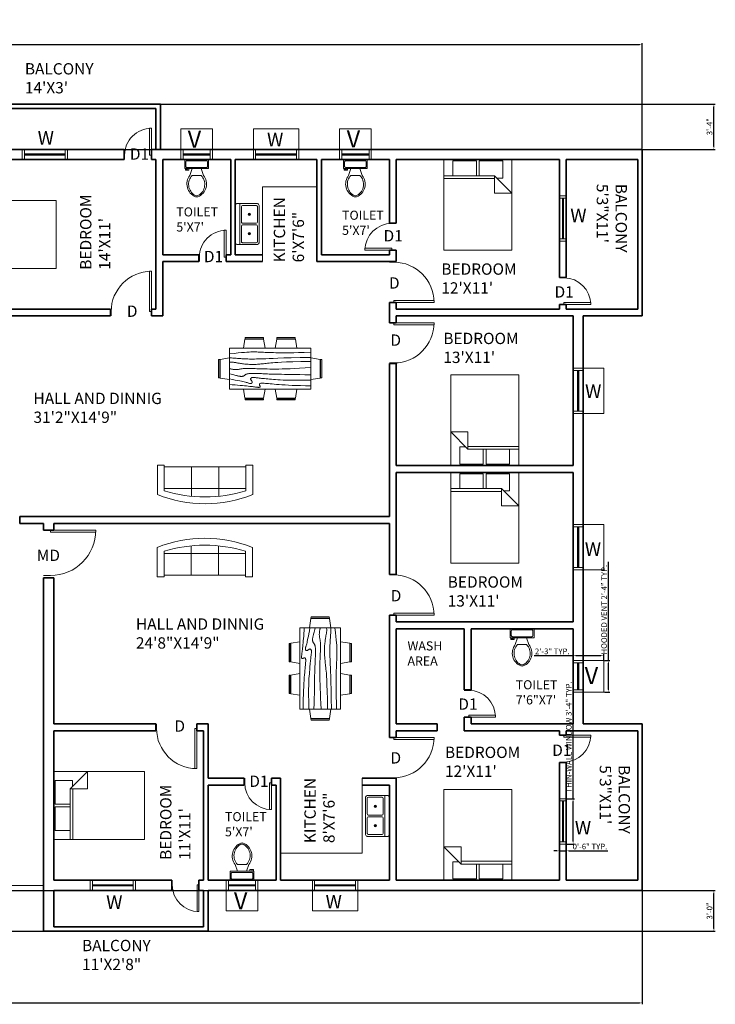
# Model space of a CAD drawing. Units: inches. Extents: x 1662 to 23131, y 1265 to 19127.
# Tile 19 of 26: x 20147 to 20761, y 18258 to 19127. Entities that reach past the tile are written whole.
import ezdxf

# ---------------------------------------------------------------- set-up
doc = ezdxf.new("R2010")
doc.units = ezdxf.units.IN
for name, color, linetype, lineweight in [('A-ANNO-DIMS', 4, 'Continuous', 18), ('A-ANNO-IDEN', 7, 'Continuous', 18), ('A-AREA-IDEN', 7, 'Continuous', 18), ('A-DOOR', 3, 'Continuous', 18), ('A-DOOR-GATE', 3, 'Continuous', 18), ('A-FLOR-CASE', 8, 'Continuous', 18), ('A-FLOR-FIXT', 9, 'Continuous', 18), ('A-FURN', 8, 'Continuous', 18), ('A-GLAZ', 4, 'Continuous', 18), ('A-WALL', 7, 'Continuous', 35)]:
    doc.layers.add(name, color=color, linetype=linetype, lineweight=lineweight)
doc.styles.get("Standard").update_dxf_attribs({"font": 'arial.ttf'})
doc.dimstyles.new('ISO-25', dxfattribs={"dimtxt": 5, "dimasz": 2.5, "dimexe": 1.25, "dimexo": 0.625, "dimtad": 1, "dimlunit": 3, "dimtxsty": 'Standard', "dimcen": 2.5, "dimadec": 0, "dimazin": 0, "dimtfac": 1, "dimtmove": 0, "dimatfit": 3, "dimfxl": 1, "dimarcsym": 0})

# ---------------------------------------------------------------- blocks, each defined once
blk = doc.blocks.new('Bed - Queen')
for p, q in [((0, -80.00003), (0, 0)), ((0, 0), (59.99999, 0)), ((59.99999, 0), (59.99999, -80.00003)), ((7.99999, -1.2), (28.79998, -1.2)), ((7.99999, -14.4), (7.99999, -1.2)), ((28.79998, -1.2), (28.79998, -14.4)), ((31.19999, -1.2), (51.99999, -1.2)), ((31.19999, -14.4), (31.19999, -1.2)), ((51.99999, -1.2), (51.99999, -16.4)), ((0, -14.4), (44.8, -14.4)), ((44.8, -16.8), (0, -16.8)), ((59.99999, -29.6), (44.8, -14.4)), ((44.8, -14.4), (44.8, -29.6)), ((51.99999, -16.4), (46.79936, -16.4)), ((44.8, -29.6), (59.99999, -29.6)), ((59.99999, -80.00003), (0, -80.00003))]:
    blk.add_line(p, q)
blk = doc.blocks.new('Toilet - top')
for p, q in [((-10, -8.5), (-8, -8.5)), ((-10, -9.5), (-10, -8.5)), ((-8, -8.5), (-8, -8)), ((-7, -8), (-7, -9.5)), ((-4, -8), (-6, -14)), ((4, -8), (6, -14)), ((9.5, -6), (9.5, -2)), ((-7, -9.5), (-10, -9.5)), ((4, -14), (-4, -14))]:
    blk.add_line(p, q)
blk.add_lwpolyline([(10.5, -8), (10.5, 0), (-10.5, 0), (-10.5, -8)], close=True)
for points in [[(-9.5, -2), (-9.5, -6)], [(8.5, -1), (-8.5, -1)], [(-8.5, -7), (8.5, -7)]]:
    blk.add_lwpolyline(points)
for centre, radius, start, end in [((-8.62, -1.88), 0.884, 81.8699, 188.1301), ((-8.62, -6.12), 0.884, 171.8699, 278.1301), ((8.62, -1.88), 0.884, 351.8699, 98.1301), ((8.62, -6.12), 0.884, 261.8699, 8.1301), ((3.52, -21.58), 12.17, 141.46911, 247.97143), ((4.2, -21.82), 11.33, 136.36773, 238.94682), ((-3.52, -21.58), 12.17, 292.02843, 38.53071), ((-4.2, -21.82), 11.33, 301.05301, 43.63209), ((0, -27.88), 4, 245.73182, 294.26817), ((0, -29), 4, 254.86053, 285.13947)]:
    blk.add_arc(centre, radius, start, end)
blk = doc.blocks.new('Sink-double - 36 in top')
for p, q in [((-18, -4), (18, -4)), ((-0.75, -18.5), (-0.75, -6.5)), ((0.75, -6.5), (0.75, -18.5))]:
    blk.add_line(p, q)
for points in [[(-16.5, 0), (16.5, 0)], [(-18, -19.5), (-18, -1.5)], [(-16.5, -18.5), (-16.5, -6.5)], [(-15.5, -5.5), (-1.75, -5.5)], [(1.75, -5.5), (15.5, -5.5)], [(16.5, -6.5), (16.5, -18.5)], [(18, -1.5), (18, -19.5)], [(16.5, -21), (-16.5, -21)], [(-1.75, -19.5), (-15.5, -19.5)], [(15.5, -19.5), (1.75, -19.5)]]:
    blk.add_lwpolyline(points)
for centre, radius in [((-8.5, -12.5), 1), ((-8.5, -12.5), 0.5), ((8.5, -12.5), 1), ((8.5, -12.5), 0.5)]:
    blk.add_circle(centre, radius)
for centre, radius, start, end in [((-16.5, -1.5), 1.5, 90, 180), ((16.5, -1.5), 1.5, 0, 90), ((-15.5, -6.5), 1, 90, 180), ((-1.75, -6.5), 1, 0, 90), ((1.75, -6.5), 1, 90, 180), ((15.5, -6.5), 1, 0, 90), ((-16.5, -19.5), 1.5, 180, 270), ((-15.5, -18.5), 1, 180, 270), ((-1.75, -18.5), 1, 270, 0), ((1.75, -18.5), 1, 180, 270), ((15.5, -18.5), 1, 270, 0), ((16.5, -19.5), 1.5, 270, 0)]:
    blk.add_arc(centre, radius, start, end)
blk = doc.blocks.new('Dining Set - 36 x 72 in.')
for p, q in [((-22, 27.5), (-22.1562, 26.50042)), ((-5.8416, 26.5), (-22.1534, 26.5)), ((-22, 27.5), (-6, 27.5)), ((-5.8437, 26.49966), (-6, 27.5)), ((6, 27.5), (5.8438, 26.50042)), ((22.1584, 26.5), (5.8466, 26.5)), ((6, 27.5), (22, 27.5)), ((22.1563, 26.49966), (22, 27.5)), ((36, 18), (-36, 18)), ((-36, 18), (-36, -18)), ((-22.2343, 26.00059), (-23.4847, 17.99762)), ((-22.2304, 26), (-5.7608, 26)), ((-4.5152, 17.99762), (-5.7655, 25.99926)), ((5.7657, 26.00059), (4.5153, 17.99762)), ((5.7696, 26), (22.2392, 26)), ((23.4848, 17.99762), (22.2345, 25.99926)), ((36, -18), (36, 18)), ((-44.0006, 8.23428), (-35.9976, 9.48474)), ((44.0006, 8.23428), (35.9976, 9.48474)), ((-45.5, 8), (-44.5004, 8.15617)), ((-45.5, 8), (-45.5, -8)), ((-44.5, -8.15843), (-44.5, 8.15338)), ((-44, 8.23041), (-44, -8.23915)), ((44, 8.23041), (44, -8.23915)), ((44.5, -8.15843), (44.5, 8.15338)), ((45.5, 8), (44.5005, 8.15617)), ((45.5, 8), (45.5, -8)), ((-44.4997, -8.15631), (-45.5, -8)), ((-35.9976, -9.48476), (-43.9993, -8.2345)), ((35.9976, -9.48476), (43.9993, -8.2345)), ((44.4997, -8.15631), (45.5, -8)), ((-36, -18), (36, -18)), ((-22.2343, -26.0006), (-23.4847, -17.99762)), ((-22.2304, -26), (-5.7608, -26)), ((-4.5152, -17.99762), (-5.7655, -25.99928)), ((5.7657, -26.0006), (4.5153, -17.99762)), ((5.7696, -26), (22.2392, -26)), ((23.4848, -17.99762), (22.2345, -25.99928)), ((-22, -27.5), (-22.1562, -26.50044)), ((-5.8416, -26.5), (-22.1534, -26.5)), ((-22, -27.5), (-6, -27.5)), ((-5.8437, -26.49967), (-6, -27.5)), ((6, -27.5), (5.8438, -26.50044)), ((22.1584, -26.5), (5.8466, -26.5)), ((6, -27.5), (22, -27.5)), ((22.1563, -26.49967), (22, -27.5))]:
    blk.add_line(p, q)
for points in [[(-36, 15), (-31.1772, 14.97754), (-26.8079, 14.91406), (-22.8538, 14.81543), (-19.276, 14.6875), (-16.0362, 14.53613), (-13.0957, 14.36718), (-10.4159, 14.18652), (-7.9583, 14), (-5.6904, 13.81315), (-3.6035, 13.63021), (-1.6954, 13.45508), (0.0365, 13.29166), (1.5945, 13.14388), (2.9811, 13.01562), (4.1988, 12.9108), (5.25, 12.83333), (6.1393, 12.78613), (6.8802, 12.76823), (7.4883, 12.77767), (7.9792, 12.8125), (8.3685, 12.87077), (8.6719, 12.95052), (8.9049, 13.0498), (9.0833, 13.16666), (9.2205, 13.29899), (9.3216, 13.44401), (9.3895, 13.59879), (9.4271, 13.76041), (9.4373, 13.92594), (9.4232, 14.09245), (9.3875, 14.257), (9.3333, 14.41666), (9.2638, 14.56917), (9.1836, 14.71484), (9.0975, 14.85465), (9.0104, 14.98958), (8.9272, 15.1206), (8.8529, 15.2487), (8.7922, 15.37483), (8.75, 15.5), (8.7305, 15.62467), (8.7344, 15.74739), (8.7617, 15.86621), (8.8125, 15.97916), (8.8867, 16.08431), (8.9844, 16.17968), (9.1055, 16.26334), (9.25, 16.33333), (9.4189, 16.38802), (9.6172, 16.42708), (9.8506, 16.45052), (10.125, 16.45833), (10.4463, 16.45052), (10.8203, 16.42708), (11.2529, 16.38802), (11.75, 16.33333), (12.3184, 16.26318), (12.9694, 16.17838), (13.7151, 16.07991), (14.5677, 15.96875), (15.5395, 15.84586), (16.6426, 15.71224), (17.8893, 15.56884), (19.2917, 15.41666), (20.859, 15.25667), (22.5879, 15.08984), (24.4721, 14.91715), (26.5052, 14.73958), (28.6809, 14.5581), (30.9929, 14.3737), (33.4347, 14.18733), (36, 14)], [(-36, 10), (-28.9766, 10.14274), (-23.1725, 10.20442), (-18.4241, 10.19775), (-14.5677, 10.13541), (-11.4399, 10.03011), (-8.877, 9.89453), (-6.7154, 9.74137), (-4.7917, 9.58333), (-2.9698, 9.43082), (-1.2246, 9.28515), (0.4415, 9.14534), (2.026, 9.01041), (3.5266, 8.87939), (4.9408, 8.7513), (6.266, 8.62516), (7.5, 8.5), (8.6411, 8.37549), (9.6914, 8.2539), (10.6538, 8.13818), (11.5312, 8.03125), (12.3267, 7.93603), (13.043, 7.85547), (13.6831, 7.79248), (14.25, 7.75), (14.7471, 7.7303), (15.1797, 7.73307), (15.5537, 7.75732), (15.875, 7.80208), (16.1494, 7.86637), (16.3828, 7.94922), (16.5811, 8.04964), (16.75, 8.16666), (16.8944, 8.29915), (17.0143, 8.44531), (17.1089, 8.60319), (17.1771, 8.77083), (17.218, 8.94629), (17.2305, 9.1276), (17.2137, 9.31282), (17.1667, 9.5), (17.0895, 9.6875), (16.987, 9.875), (16.8649, 10.0625), (16.7292, 10.25), (16.5856, 10.4375), (16.4401, 10.625), (16.2985, 10.8125), (16.1667, 11), (16.05, 11.18733), (15.9518, 11.3737), (15.8752, 11.5581), (15.8229, 11.73958), (15.798, 11.91715), (15.8034, 12.08984), (15.842, 12.25667), (15.9167, 12.41666), (16.0295, 12.56836), (16.1784, 12.70833), (16.3605, 12.83268), (16.5729, 12.9375), (16.8127, 13.01888), (17.0768, 13.07291), (17.3625, 13.0957), (17.6667, 13.08333), (17.9894, 13.03312), (18.3418, 12.94726), (18.7382, 12.82918), (19.1927, 12.68229), (19.7195, 12.51001), (20.3327, 12.31575), (21.0465, 12.10294), (21.875, 11.875), (22.8357, 11.63354), (23.959, 11.37304), (25.2786, 11.08618), (26.8282, 10.76562), (28.6414, 10.40405), (30.752, 9.99414), (33.1936, 9.52856), (36, 9)], [(-36, 5.5), (-30.7157, 5.3348), (-26.069, 5.20963), (-21.9946, 5.11767), (-18.4271, 5.05208), (-15.3009, 5.00602), (-12.5508, 4.97265), (-10.1112, 4.94515), (-7.9167, 4.91666), (-5.909, 4.88167), (-4.0586, 4.83984), (-2.3429, 4.79215), (-0.7396, 4.73958), (0.7739, 4.6831), (2.22, 4.6237), (3.6213, 4.56233), (5, 4.5), (6.373, 4.43782), (7.7344, 4.3776), (9.0723, 4.32129), (10.375, 4.27083), (11.6309, 4.22819), (12.8281, 4.19531), (13.9551, 4.17415), (15, 4.16666), (15.954, 4.17448), (16.819, 4.19791), (17.6001, 4.23698), (18.3021, 4.29166), (18.9299, 4.36198), (19.4883, 4.44791), (19.9823, 4.54948), (20.4167, 4.66666), (20.7969, 4.79899), (21.1302, 4.94401), (21.4245, 5.09879), (21.6875, 5.26041), (21.9271, 5.42594), (22.1511, 5.59245), (22.3672, 5.757), (22.5834, 5.91666), (22.8065, 6.06868), (23.0404, 6.21093), (23.2879, 6.34147), (23.5521, 6.45833), (23.8358, 6.55957), (24.142, 6.64323), (24.4735, 6.70735), (24.8334, 6.75), (25.2235, 6.76969), (25.642, 6.76692), (26.0858, 6.74267), (26.5521, 6.69791), (27.0379, 6.63362), (27.5404, 6.55078), (28.0565, 6.45036), (28.5834, 6.33333), (29.1242, 6.19987), (29.7071, 6.04687), (30.3661, 5.87044), (31.1354, 5.66666), (32.0493, 5.43164), (33.142, 5.16146), (34.4475, 4.85221), (36, 4.5)], [(-36, -1), (-30.7915, -0.6591), (-26.0195, -0.38216), (-21.6519, -0.16284), (-17.6563, 0.00521), (-14.0005, 0.12833), (-10.6523, 0.21289), (-7.5796, 0.26522), (-4.75, 0.29166), (-2.134, 0.29793), (0.2878, 0.28711), (2.5317, 0.26163), (4.6146, 0.22396), (6.5529, 0.17651), (8.3633, 0.12174), (10.0623, 0.06209), (11.6667, 0), (13.1899, -0.06201), (14.6341, -0.1211), (15.9982, -0.17432), (17.2813, -0.21875), (18.4823, -0.25147), (19.6003, -0.26953), (20.6343, -0.27002), (21.5834, -0.25), (22.4481, -0.20768), (23.2357, -0.14584), (23.9549, -0.06836), (24.6146, 0.02083), (25.2235, 0.11784), (25.7904, 0.21875), (26.3241, 0.31966), (26.8334, 0.41666), (27.3265, 0.50618), (27.8099, 0.58593), (28.2894, 0.65397), (28.7709, 0.70833), (29.2601, 0.74707), (29.763, 0.76823), (30.2855, 0.76985), (30.8334, 0.75), (31.4088, 0.70784), (31.9994, 0.64713), (32.589, 0.57275), (33.1615, 0.48958), (33.7008, 0.4025), (34.1908, 0.3164), (34.6153, 0.23616), (34.9584, 0.16666), (35.2099, 0.11165), (35.3848, 0.07031), (35.504, 0.04069), (35.5886, 0.02083), (35.6594, 0.00879), (35.7377, 0.0026), (35.8442, 0.00032), (36, 0)], [(-36, -6.5), (-27.1843, -6.31267), (-20.084, -6.1263), (-14.469, -5.9419), (-10.1094, -5.76042), (-6.7752, -5.58285), (-4.2363, -5.41016), (-2.2629, -5.24333), (-0.625, -5.08334), (0.8708, -4.93099), (2.2715, -4.78646), (3.5872, -4.64974), (4.8281, -4.52084), (6.0046, -4.39974), (7.127, -4.28646), (8.2053, -4.18099), (9.25, -4.08334), (10.2705, -3.99382), (11.2734, -3.91407), (12.2647, -3.84603), (13.25, -3.79167), (14.2354, -3.75293), (15.2266, -3.73177), (16.2295, -3.73015), (17.25, -3.75), (18.2912, -3.79248), (19.3451, -3.85547), (20.4009, -3.93604), (21.4479, -4.03125), (22.4754, -4.13819), (23.4727, -4.25391), (24.4289, -4.37549), (25.3334, -4.5), (26.1785, -4.62492), (26.9694, -4.74935), (27.7145, -4.87281), (28.4219, -4.99479), (29.1, -5.11483), (29.7572, -5.23242), (30.4016, -5.34709), (31.0417, -5.45834), (31.6837, -5.56437), (32.3262, -5.65821), (32.9658, -5.73153), (33.599, -5.77604), (34.2224, -5.78345), (34.8327, -5.74545), (35.4264, -5.65373), (36, -5.5)], [(-36, -10), (-26.4022, -9.81299), (-18.4675, -9.62891), (-11.9839, -9.45069), (-6.7396, -9.28125), (-2.5226, -9.12354), (0.8789, -8.98047), (3.6769, -8.85498), (6.0833, -8.75), (8.2767, -8.66765), (10.3021, -8.60677), (12.1712, -8.56543), (13.8958, -8.54167), (15.4876, -8.53353), (16.9583, -8.53907), (18.3197, -8.55632), (19.5834, -8.58334), (20.7616, -8.61841), (21.8685, -8.66081), (22.9188, -8.71004), (23.9271, -8.76563), (24.9081, -8.82707), (25.8763, -8.89388), (26.8465, -8.96558), (27.8334, -9.04167), (28.8474, -9.12118), (29.8828, -9.20117), (30.93, -9.27824), (31.9792, -9.34896), (33.0205, -9.40991), (34.0443, -9.45768), (35.0407, -9.48885), (36, -9.5)], [(-36, -14.5), (-30.0881, -14.33513), (-25.0332, -14.21224), (-20.7312, -14.12647), (-17.0781, -14.07292), (-13.97, -14.04671), (-11.3027, -14.04297), (-8.9724, -14.05681), (-6.875, -14.08334), (-4.9224, -14.11833), (-3.0905, -14.16016), (-1.3709, -14.20785), (0.2448, -14.26042), (1.7647, -14.3169), (3.1973, -14.3763), (4.5507, -14.43767), (5.8333, -14.5), (7.0554, -14.5621), (8.235, -14.62175), (9.3922, -14.67652), (10.5469, -14.72396), (11.7192, -14.76164), (12.929, -14.78711), (14.1965, -14.79794), (15.5417, -14.79167), (16.9933, -14.76424), (18.6152, -14.70508), (20.4804, -14.60197), (22.6615, -14.44271), (25.2312, -14.21509), (28.2624, -13.9069), (31.8277, -13.50594), (36, -13)]]:
    blk.add_lwpolyline(points)
blk = doc.blocks.new('Sofa - Roundback 7 ft.')
for p, q in [((-12.00002, -32.4421), (-12.00003, -6.5971)), ((11.99997, -32.4421), (11.99998, -6.5971)), ((-36.000027, -34), (-36.000027, -11.4696)), ((-35.999844, -13.3819), (35.9998, -13.3819)), ((35.99998, -34), (35.99998, -11.4696)), ((-36.000027, -32.4421), (35.99998, -32.4421))]:
    blk.add_line(p, q)
for points in [[(-36.000027, -34), (-42.000027, -34), (-42.000027, -8)], [(41.99998, -8), (41.99998, -34), (35.99998, -34)]]:
    blk.add_lwpolyline(points)
for centre, radius, start, end in [((0, -114.25), 114.25, 68.43141, 111.5686), ((-0.00001, -127.1968), 121.1968, 72.72033, 107.2797)]:
    blk.add_arc(centre, radius, start, end)
blk = doc.blocks.new('*U4')
for p, q in [((0, 0), (0, -100)), ((-900, 0), (-900, -100))]:
    blk.add_line(p, q)
blk.add_lwpolyline([(0, 0), (0, 900), (-43.75, 900), (-43.75, 0)], close=True)
blk.add_arc((0, 0), 900, 90, 180)
blk = doc.blocks.new('*U100')
for p, q in [((-900, 0), (-900, 100)), ((0, 0), (0, 100))]:
    blk.add_line(p, q)
blk.add_lwpolyline([(0, 0), (0, -900), (-43.75, -900), (-43.75, 0)], close=True)
blk.add_arc((0, 0), 900, 180, 270)
blk = doc.blocks.new('*U101')
for p, q in [((0, 0), (0, -100)), ((900, 0), (900, -100))]:
    blk.add_line(p, q)
blk.add_lwpolyline([(0, 0), (0, 900), (43.75, 900), (43.75, 0)], close=True)
blk.add_arc((0, 0), 900, 0, 90)
blk = doc.blocks.new('*U103')
for p, q in [((0, 0), (0, -100)), ((600, 0), (600, -100))]:
    blk.add_line(p, q)
blk.add_lwpolyline([(0, 0), (0, 600), (43.75, 600), (43.75, 0)], close=True)
blk.add_arc((0, 0), 600, 0, 90)
blk = doc.blocks.new('*U105')
for p, q in [((-600, 0), (-600, -100)), ((0, 0), (0, -100))]:
    blk.add_line(p, q)
blk.add_lwpolyline([(0, 0), (0, 600), (-43.75, 600), (-43.75, 0)], close=True)
blk.add_arc((0, 0), 600, 90, 180)
blk = doc.blocks.new('*U104')
for p, q in [((-600, 0), (-600, -100)), ((0, 0), (0, -100))]:
    blk.add_line(p, q)
blk.add_lwpolyline([(0, 0), (0, 600), (-43.75, 600), (-43.75, 0)], close=True)
blk.add_arc((0, 0), 600, 90, 180)
blk = doc.blocks.new('*U106')
for p, q in [((-600, 0), (-600, 100)), ((0, 0), (0, 100))]:
    blk.add_line(p, q)
blk.add_lwpolyline([(0, 0), (0, -600), (-43.75, -600), (-43.75, 0)], close=True)
blk.add_arc((0, 0), 600, 180, 270)
blk = doc.blocks.new('*U107')
for p, q in [((0, 0), (0, 100)), ((600, 0), (600, 100))]:
    blk.add_line(p, q)
blk.add_lwpolyline([(0, 0), (0, -600), (43.75, -600), (43.75, 0)], close=True)
blk.add_arc((0, 0), 600, 270, 0)
blk = doc.blocks.new('*U108')
for p, q in [((0, 0), (0, -100)), ((600, 0), (600, -100))]:
    blk.add_line(p, q)
blk.add_lwpolyline([(0, 0), (0, 600), (43.75, 600), (43.75, 0)], close=True)
blk.add_arc((0, 0), 600, 0, 90)
blk = doc.blocks.new('*U113')
for p, q in [((0, 0), (0, -6)), ((40, 0), (40, -6))]:
    blk.add_line(p, q)
blk.add_lwpolyline([(0, 0), (0, 40), (1.75, 40), (1.75, 0)], close=True)
blk.add_arc((0, 0), 40, 0, 90)
blk = doc.blocks.new('*D115')
at = {"layer": 'A-ANNO-DIMS', "color": 0, "lineweight": -2, "transparency": 16777216}
for p, q in [((19495.19, 19013.32), (19495.19, 19106.49)), ((19497.69, 19105.24), (20693.69, 19105.24)), ((20696.19, 19013.32), (20696.19, 19106.49))]:
    blk.add_line(p, q, dxfattribs=at)
at = {"layer": 'A-ANNO-DIMS', "color": 0, "transparency": 16777216}
for points in [[(19497.69, 19105.65), (19497.69, 19104.82), (19495.19, 19105.24)], [(20693.69, 19105.65), (20693.69, 19104.82), (20696.19, 19105.24)]]:
    blk.add_solid(points, dxfattribs=at)
at = {"layer": 'Defpoints', "color": 0, "transparency": 16777216}
for p in [(20696.19, 19105.24), (19495.19, 19012.7), (20696.19, 19012.7)]:
    blk.add_point(p, dxfattribs=at)
at = {"layer": 'A-ANNO-DIMS', "color": 0, "transparency": 16777216, "insert": (20095.69, 19116.07), "char_height": 5, "attachment_point": 5}
blk.add_mtext('{\\H4x;100\'-1"}', dxfattribs=at)
blk = doc.blocks.new('WIN-36-J9X2')
for p, q in [((0, 0), (0, 9)), ((2, 0), (2, 9)), ((38, 0), (38, 9)), ((40, 0), (40, 9)), ((38, 5), (2, 5)), ((38, 4.5), (2, 4.5)), ((38, 4), (2, 4))]:
    blk.add_line(p, q)
blk = doc.blocks.new('WIN-36-J9X2-HOOD')
for p, q in [((0, 27), (0, 18)), ((2, 27), (2, 18)), ((38, 27), (38, 18)), ((40, 27), (40, 18)), ((0, 18), (0, 0)), ((2, 23), (38, 23)), ((2, 22.5), (38, 22.5)), ((2, 22), (38, 22)), ((40, 0), (40, 18)), ((0, 0), (40, 0))]:
    blk.add_line(p, q)
blk = doc.blocks.new('WIN-36-J6X2')
for p, q in [((6, 40), (0, 40)), ((6, 38), (0, 38)), ((2.5, 38), (2.5, 2)), ((3, 38), (3, 2)), ((3.5, 38), (3.5, 2)), ((6, 2), (0, 2)), ((6, 0), (0, 0))]:
    blk.add_line(p, q)
blk = doc.blocks.new('VENT-24-J9X2-HOOD')
for p, q in [((0, 18), (0, 27)), ((2, 18), (2, 27)), ((26, 18), (26, 27)), ((28, 18), (28, 27)), ((0, 18), (0, 0)), ((26, 23), (2, 23)), ((26, 22.5), (2, 22.5)), ((26, 22), (2, 22)), ((28, 0), (28, 18)), ((0, 0), (28, 0))]:
    blk.add_line(p, q)
blk = doc.blocks.new('*D175')
at = {"layer": 'A-ANNO-DIMS', "color": 0, "lineweight": -2, "transparency": 16777216}
for p, q in [((20666.39, 18561.7), (20666.39, 18648.82)), ((20662.82, 18561.7), (20667.64, 18561.7)), ((20666.39, 18536.2), (20666.39, 18559.2)), ((20662.82, 18533.7), (20667.64, 18533.7))]:
    blk.add_line(p, q, dxfattribs=at)
at = {"layer": 'A-ANNO-DIMS', "color": 0, "transparency": 16777216}
for points in [[(20665.98, 18559.2), (20666.81, 18559.2), (20666.39, 18561.7)], [(20665.98, 18536.2), (20666.81, 18536.2), (20666.39, 18533.7)]]:
    blk.add_solid(points, dxfattribs=at)
at = {"layer": 'Defpoints', "color": 0, "transparency": 16777216}
for p in [(20662.19, 18561.7), (20666.39, 18561.7), (20662.19, 18533.7)]:
    blk.add_point(p, dxfattribs=at)
at = {"layer": 'A-ANNO-DIMS', "color": 0, "transparency": 16777216, "insert": (20663.18, 18606.51), "char_height": 5, "attachment_point": 5, "rotation": 90}
blk.add_mtext('HOODED VENT 2\'-4" TYP.', dxfattribs=at)
blk = doc.blocks.new('*D176')
at = {"layer": 'A-ANNO-DIMS', "color": 0, "lineweight": -2, "transparency": 16777216}
for p, q in [((20635.19, 18562.32), (20635.19, 18567.15)), ((20662.19, 18562.32), (20662.19, 18567.15)), ((20635.19, 18565.9), (20600.88, 18565.9)), ((20659.69, 18565.9), (20637.69, 18565.9))]:
    blk.add_line(p, q, dxfattribs=at)
at = {"layer": 'A-ANNO-DIMS', "color": 0, "transparency": 16777216}
for points in [[(20637.69, 18566.31), (20637.69, 18565.48), (20635.19, 18565.9)], [(20659.69, 18566.31), (20659.69, 18565.48), (20662.19, 18565.9)]]:
    blk.add_solid(points, dxfattribs=at)
at = {"layer": 'Defpoints', "color": 0, "transparency": 16777216}
for p in [(20635.19, 18565.9), (20635.19, 18561.7), (20662.19, 18561.7)]:
    blk.add_point(p, dxfattribs=at)
at = {"layer": 'A-ANNO-DIMS', "color": 0, "transparency": 16777216, "insert": (20616.79, 18569.08), "char_height": 5, "attachment_point": 5}
blk.add_mtext('2\'-3" TYP.', dxfattribs=at)
blk = doc.blocks.new('*D191')
at = {"layer": 'A-ANNO-DIMS', "color": 0, "lineweight": -2, "transparency": 16777216}
for p, q in [((20635.19, 18439.7), (20635.19, 18546.22)), ((20629.82, 18439.7), (20636.44, 18439.7)), ((20635.19, 18402.2), (20635.19, 18437.2)), ((20629.82, 18399.7), (20636.44, 18399.7))]:
    blk.add_line(p, q, dxfattribs=at)
at = {"layer": 'A-ANNO-DIMS', "color": 0, "transparency": 16777216}
for points in [[(20634.78, 18437.2), (20635.61, 18437.2), (20635.19, 18439.7)], [(20634.78, 18402.2), (20635.61, 18402.2), (20635.19, 18399.7)]]:
    blk.add_solid(points, dxfattribs=at)
at = {"layer": 'Defpoints', "color": 0, "transparency": 16777216}
for p in [(20629.19, 18439.7), (20635.19, 18439.7), (20629.19, 18399.7)]:
    blk.add_point(p, dxfattribs=at)
at = {"layer": 'A-ANNO-DIMS', "color": 0, "transparency": 16777216, "insert": (20631.98, 18494.21), "char_height": 5, "attachment_point": 5, "rotation": 90}
blk.add_mtext('THIN-WALL WINDOW 3\'-4" TYP.', dxfattribs=at)
blk = doc.blocks.new('*D192')
at = {"layer": 'A-ANNO-DIMS', "color": 0, "lineweight": -2, "transparency": 16777216}
for p, q in [((20620.69, 18393.7), (20618.19, 18393.7)), ((20623.19, 18399.07), (20623.19, 18392.45)), ((20623.19, 18393.7), (20629.19, 18393.7)), ((20629.19, 18399.07), (20629.19, 18392.45)), ((20631.69, 18393.7), (20665.92, 18393.7))]:
    blk.add_line(p, q, dxfattribs=at)
at = {"layer": 'A-ANNO-DIMS', "color": 0, "transparency": 16777216}
for points in [[(20620.69, 18394.11), (20620.69, 18393.28), (20623.19, 18393.7)], [(20631.69, 18394.11), (20631.69, 18393.28), (20629.19, 18393.7)]]:
    blk.add_solid(points, dxfattribs=at)
at = {"layer": 'Defpoints', "color": 0, "transparency": 16777216}
for p in [(20623.19, 18399.7), (20629.19, 18399.7), (20629.19, 18393.7)]:
    blk.add_point(p, dxfattribs=at)
at = {"layer": 'A-ANNO-DIMS', "color": 0, "transparency": 16777216, "insert": (20650.06, 18396.87), "char_height": 5, "attachment_point": 5}
blk.add_mtext('0\'-6" TYP.', dxfattribs=at)
blk = doc.blocks.new('*D251')
at = {"layer": 'A-ANNO-DIMS', "color": 0, "lineweight": -2, "transparency": 16777216}
for p, q in [((19491.19, 18358.07), (19491.19, 18258.3)), ((20696.19, 18358.07), (20696.19, 18258.3)), ((19493.69, 18259.55), (20693.69, 18259.55))]:
    blk.add_line(p, q, dxfattribs=at)
at = {"layer": 'A-ANNO-DIMS', "color": 0, "transparency": 16777216}
for points in [[(19493.69, 18259.96), (19493.69, 18259.13), (19491.19, 18259.55)], [(20693.69, 18259.96), (20693.69, 18259.13), (20696.19, 18259.55)]]:
    blk.add_solid(points, dxfattribs=at)
at = {"layer": 'Defpoints', "color": 0, "transparency": 16777216}
for p in [(19491.19, 18358.7), (20696.19, 18358.7), (20696.19, 18259.55)]:
    blk.add_point(p, dxfattribs=at)
at = {"layer": 'A-ANNO-DIMS', "color": 0, "transparency": 16777216, "insert": (20093.69, 18262.72), "char_height": 5, "attachment_point": 5}
blk.add_mtext('100\'-5"', dxfattribs=at)
blk = doc.blocks.new('*D252')
at = {"layer": 'A-ANNO-DIMS', "color": 0, "lineweight": -2, "transparency": 16777216}
for p, q in [((19918.82, 19052.7), (20760.59, 19052.7)), ((20759.34, 19015.2), (20759.34, 19050.2)), ((19918.82, 19012.7), (20760.59, 19012.7))]:
    blk.add_line(p, q, dxfattribs=at)
at = {"layer": 'A-ANNO-DIMS', "color": 0, "transparency": 16777216}
for points in [[(20758.93, 19050.2), (20759.76, 19050.2), (20759.34, 19052.7)], [(20758.93, 19015.2), (20759.76, 19015.2), (20759.34, 19012.7)]]:
    blk.add_solid(points, dxfattribs=at)
at = {"layer": 'Defpoints', "color": 0, "transparency": 16777216}
for p in [(19918.19, 19052.7), (20759.34, 19052.7), (19918.19, 19012.7)]:
    blk.add_point(p, dxfattribs=at)
at = {"layer": 'A-ANNO-DIMS', "color": 0, "transparency": 16777216, "insert": (20756.16, 19032.7), "char_height": 5, "attachment_point": 5, "rotation": 90}
blk.add_mtext('3\'-4"', dxfattribs=at)
blk = doc.blocks.new('*D253')
at = {"layer": 'A-ANNO-DIMS', "color": 0, "lineweight": -2, "transparency": 16777216}
for p, q in [((19996.82, 18358.7), (20760.59, 18358.7)), ((20759.34, 18325.2), (20759.34, 18356.2)), ((19996.82, 18322.7), (20760.59, 18322.7))]:
    blk.add_line(p, q, dxfattribs=at)
at = {"layer": 'A-ANNO-DIMS', "color": 0, "transparency": 16777216}
for points in [[(20758.93, 18356.2), (20759.76, 18356.2), (20759.34, 18358.7)], [(20758.93, 18325.2), (20759.76, 18325.2), (20759.34, 18322.7)]]:
    blk.add_solid(points, dxfattribs=at)
at = {"layer": 'Defpoints', "color": 0, "transparency": 16777216}
for p in [(19996.19, 18358.7), (20759.34, 18358.7), (19996.19, 18322.7)]:
    blk.add_point(p, dxfattribs=at)
at = {"layer": 'A-ANNO-DIMS', "color": 0, "transparency": 16777216, "insert": (20756.16, 18340.7), "char_height": 5, "attachment_point": 5, "rotation": 90}
blk.add_mtext('3\'-0"', dxfattribs=at)

msp = doc.modelspace()

# ---------------------------------------------------------------- linework, layer by layer
at = {"layer": 'A-DOOR-GATE'}
msp.add_line((20099.192, 18363.196), (20168.192, 18363.196), dxfattribs=at)
at = {"layer": 'A-FLOR-CASE'}
for p, q in [((20361.192, 18913.696), (20361.192, 18979.696)), ((20361.192, 18979.696), (20409.192, 18979.696)), ((20449.192, 18391.696), (20449.192, 18457.696)), ((20377.192, 18391.696), (20449.192, 18391.696))]:
    msp.add_line(p, q, dxfattribs=at)
at = {"layer": 'A-WALL'}
for p, q in [((19918.192, 19052.696), (20271.192, 19052.696)), ((20099.192, 19048.696), (20267.192, 19048.696)), ((20267.192, 19048.696), (20267.192, 19012.696)), ((20271.192, 19052.696), (20271.192, 19012.696)), ((20099.192, 19012.696), (20239.192, 19012.696)), ((20239.192, 19003.696), (20239.192, 19012.696)), ((20263.192, 19003.696), (20263.192, 19012.696)), ((20263.192, 19012.696), (20696.192, 19012.696)), ((20696.192, 18865.696), (20696.192, 19012.696)), ((20099.192, 19003.696), (20239.192, 19003.696)), ((20263.192, 19003.696), (20267.192, 19003.696)), ((20267.192, 18871.696), (20267.192, 19003.696)), ((20273.192, 18919.696), (20273.192, 19003.696)), ((20273.192, 19003.696), (20333.192, 19003.696)), ((20333.192, 18919.696), (20333.192, 19003.696)), ((20337.192, 18919.696), (20337.192, 19003.696)), ((20337.192, 19003.696), (20409.192, 19003.696)), ((20409.192, 18913.696), (20409.192, 19003.696)), ((20413.192, 18919.696), (20413.192, 19003.696)), ((20413.192, 19003.696), (20473.192, 19003.696)), ((20473.192, 18947.696), (20473.192, 19003.696)), ((20479.192, 18947.696), (20479.192, 19003.696)), ((20479.192, 19003.696), (20623.192, 19003.696)), ((20623.192, 18899.696), (20623.192, 19003.696)), ((20629.192, 18899.696), (20629.192, 19003.696)), ((20629.192, 19003.696), (20692.192, 19003.696)), ((20692.192, 18871.696), (20692.192, 19003.696)), ((20337.192, 18946.786), (20337.192, 18946.786)), ((20473.192, 18947.696), (20479.192, 18947.696)), ((20473.192, 18923.696), (20479.192, 18923.696)), ((20473.192, 18919.696), (20473.192, 18923.696)), ((20479.192, 18913.696), (20479.192, 18923.696)), ((20273.192, 18919.696), (20305.192, 18919.696)), ((20305.192, 18919.696), (20305.192, 18913.696)), ((20329.192, 18919.696), (20329.192, 18913.696)), ((20329.192, 18919.696), (20333.192, 18919.696)), ((20337.192, 18919.696), (20361.192, 18919.696)), ((20413.192, 18919.696), (20473.192, 18919.696)), ((20273.192, 18865.696), (20273.192, 18913.696)), ((20273.192, 18913.696), (20305.192, 18913.696)), ((20329.192, 18913.696), (20361.192, 18913.696)), ((20409.192, 18913.696), (20473.192, 18913.696)), ((20479.192, 18913.696), (20473.192, 18913.696)), ((20629.192, 18899.696), (20623.192, 18899.696)), ((20099.192, 18871.696), (20227.192, 18871.696)), ((20227.192, 18865.696), (20227.192, 18871.696)), ((20263.192, 18865.696), (20263.192, 18871.696)), ((20263.192, 18871.696), (20267.192, 18871.696)), ((20479.192, 18877.696), (20473.192, 18877.696)), ((20473.192, 18859.696), (20473.192, 18877.696)), ((20479.192, 18871.696), (20479.192, 18877.696)), ((20479.192, 18871.696), (20623.192, 18871.696)), ((20623.192, 18871.696), (20479.192, 18871.696)), ((20623.192, 18871.696), (20623.192, 18875.696)), ((20629.192, 18875.696), (20623.192, 18875.696)), ((20629.192, 18871.696), (20629.192, 18875.696)), ((20692.192, 18871.696), (20629.192, 18871.696)), ((20629.192, 18871.696), (20635.192, 18871.696)), ((20099.192, 18865.696), (20227.192, 18865.696)), ((20263.192, 18865.696), (20273.192, 18865.696)), ((20635.192, 18865.696), (20479.192, 18865.696)), ((20479.192, 18865.696), (20635.192, 18865.696)), ((20479.192, 18859.696), (20479.192, 18865.696)), ((20635.192, 18733.696), (20635.192, 18865.696)), ((20644.192, 18505.696), (20644.192, 18865.696)), ((20644.192, 18865.696), (20696.192, 18865.696)), ((20479.192, 18859.696), (20473.192, 18859.696)), ((20479.192, 18823.696), (20473.192, 18823.696)), ((20473.192, 18688.696), (20473.192, 18823.696)), ((20479.192, 18733.696), (20479.192, 18823.696)), ((20635.192, 18733.696), (20479.192, 18733.696)), ((20635.192, 18727.696), (20479.192, 18727.696)), ((20479.192, 18637.696), (20479.192, 18727.696)), ((20635.192, 18595.696), (20635.192, 18727.696)), ((20147.192, 18682.696), (20147.192, 18688.696)), ((20147.192, 18688.696), (20473.192, 18688.696)), ((20147.192, 18682.696), (20168.192, 18682.696)), ((20168.192, 18676.696), (20168.192, 18682.696)), ((20177.192, 18682.696), (20473.192, 18682.696)), ((20177.192, 18676.696), (20177.192, 18682.696)), ((20177.192, 18682.696), (20267.617, 18682.696)), ((20473.192, 18637.696), (20473.192, 18682.696)), ((20168.192, 18676.696), (20177.192, 18676.696)), ((20473.192, 18637.696), (20479.192, 18637.696)), ((20168.192, 18505.696), (20168.192, 18634.696)), ((20168.192, 18634.696), (20177.192, 18634.696)), ((20177.192, 18505.696), (20177.192, 18634.696)), ((20473.192, 18601.696), (20479.192, 18601.696)), ((20473.192, 18493.696), (20473.192, 18601.696)), ((20479.192, 18595.696), (20479.192, 18601.696)), ((20168.192, 18599.18), (20168.192, 18322.696)), ((20168.192, 18367.696), (20168.192, 18599.18)), ((20479.192, 18595.696), (20635.192, 18595.696)), ((20479.192, 18589.696), (20539.192, 18589.696)), ((20479.192, 18505.696), (20479.192, 18589.696)), ((20539.192, 18535.696), (20539.192, 18589.696)), ((20545.192, 18589.696), (20635.192, 18589.696)), ((20545.192, 18535.696), (20545.192, 18589.696)), ((20635.192, 18505.696), (20635.192, 18589.696)), ((20539.192, 18535.696), (20545.192, 18535.696)), ((20539.192, 18499.696), (20539.192, 18511.696)), ((20539.192, 18511.696), (20545.192, 18511.696)), ((20545.192, 18505.696), (20545.192, 18511.696)), ((20177.192, 18505.696), (20267.192, 18505.696)), ((20177.192, 18367.696), (20177.192, 18499.696)), ((20177.192, 18499.696), (20267.192, 18499.696)), ((20267.192, 18499.696), (20267.192, 18505.696)), ((20303.192, 18499.696), (20303.192, 18505.696)), ((20303.192, 18505.696), (20313.192, 18505.696)), ((20303.192, 18499.696), (20309.192, 18499.696)), ((20309.192, 18367.696), (20309.192, 18499.696)), ((20313.192, 18457.696), (20313.192, 18505.696)), ((20479.192, 18505.696), (20515.192, 18505.696)), ((20479.192, 18499.696), (20515.192, 18499.696)), ((20479.192, 18493.696), (20479.192, 18499.696)), ((20515.192, 18499.696), (20515.192, 18505.696)), ((20539.192, 18499.696), (20623.192, 18499.696)), ((20545.192, 18505.696), (20635.192, 18505.696)), ((20623.192, 18495.696), (20623.192, 18499.696)), ((20629.192, 18495.696), (20629.192, 18499.696)), ((20629.192, 18499.696), (20692.192, 18499.696)), ((20644.192, 18505.696), (20696.192, 18505.696)), ((20692.192, 18499.696), (20692.192, 18367.696)), ((20696.192, 18505.696), (20696.192, 18358.696)), ((20473.192, 18493.696), (20479.192, 18493.696)), ((20623.192, 18495.696), (20629.192, 18495.696)), ((20623.192, 18367.696), (20623.192, 18471.696)), ((20623.192, 18471.696), (20629.192, 18471.696)), ((20629.192, 18367.696), (20629.192, 18471.696)), ((20313.192, 18457.696), (20345.192, 18457.696)), ((20345.192, 18451.696), (20345.192, 18457.696)), ((20369.192, 18451.696), (20369.192, 18457.696)), ((20369.192, 18457.696), (20377.192, 18457.696)), ((20377.192, 18367.696), (20377.192, 18457.696)), ((20449.192, 18457.696), (20479.192, 18457.696)), ((20479.192, 18367.696), (20479.192, 18457.696)), ((20313.192, 18367.696), (20313.192, 18451.696)), ((20313.192, 18451.696), (20345.192, 18451.696)), ((20369.192, 18451.696), (20373.192, 18451.696)), ((20373.192, 18367.696), (20373.192, 18451.696)), ((20449.192, 18451.696), (20473.192, 18451.696)), ((20473.192, 18367.696), (20473.192, 18451.696)), ((20177.192, 18367.696), (20281.192, 18367.696)), ((20281.192, 18358.696), (20281.192, 18367.696)), ((20305.192, 18358.696), (20305.192, 18367.696)), ((20305.192, 18367.696), (20309.192, 18367.696)), ((20313.192, 18367.696), (20373.192, 18367.696)), ((20377.192, 18367.696), (20473.192, 18367.696)), ((20479.192, 18367.696), (20623.192, 18367.696)), ((20629.192, 18367.696), (20692.192, 18367.696)), ((20177.192, 18358.696), (20177.192, 18326.696)), ((20177.192, 18358.696), (20281.192, 18358.696)), ((20305.192, 18358.696), (20309.192, 18358.696)), ((20309.192, 18326.696), (20309.192, 18358.696)), ((20313.192, 18322.696), (20313.192, 18358.696)), ((20313.192, 18358.696), (20696.192, 18358.696)), ((20177.192, 18326.696), (20309.192, 18326.696)), ((20168.192, 18322.696), (20313.192, 18322.696))]:
    msp.add_line(p, q, dxfattribs=at)

# ---------------------------------------------------------------- block references
at = {"layer": 'A-DOOR', "xscale": 0.0393700787401575, "yscale": 0.0393700787401575, "zscale": 0.0393700787401575}
for name, p, rotation in [('*U107', (20263.192, 19007.633), 180), ('*U107', (20329.192, 18917.633), 180), ('*U106', (20475.255, 18923.696), 270), ('*U4', (20477.129, 18877.696), 270), ('*U105', (20627.129, 18875.696), 270), ('*U101', (20477.129, 18859.696), 270), ('*U4', (20477.129, 18601.696), 270), ('*U104', (20543.129, 18511.696), 270), ('*U101', (20477.129, 18493.696), 270), ('*U103', (20627.129, 18495.696), 270), ('*U108', (20369.192, 18453.759), 180), ('*U108', (20305.192, 18363.759), 180)]:
    msp.add_blockref(name, p, dxfattribs=dict(at, rotation=rotation))
for name, p in [('*U4', (20263.192, 18869.633)), ('*U100', (20303.192, 18501.759))]:
    msp.add_blockref(name, p, dxfattribs=at)
at = {"layer": 'A-DOOR', "rotation": 270}
msp.add_blockref('*U113', (20174.192, 18676.696), dxfattribs=at)
at = {"layer": 'A-FLOR-FIXT'}
for p in [(20303.192, 19003.696), (20443.192, 19003.696), (20590.192, 18589.696)]:
    msp.add_blockref('Toilet - top', p, dxfattribs=at)
for name, p, rotation in [('Sink-double - 36 in top', (20337.192, 18946.786), 89.99999999999999), ('Sink-double - 36 in top', (20473.192, 18424.502), 270), ('Toilet - top', (20343.192, 18367.696), 180)]:
    msp.add_blockref(name, p, dxfattribs=dict(at, rotation=rotation))
at = {"layer": 'A-FURN'}
for name, p in [('Bed - Queen', (20521.192, 19003.696)), ('Bed - Queen', (20527.192, 18727.696)), ('Sofa - Roundback 7 ft.', (20310.359, 18669.467))]:
    msp.add_blockref(name, p, dxfattribs=at)
for name, p, rotation in [('Bed - Queen', (20099.192, 18907.696), 89.99999999999999), ('Dining Set - 36 x 72 in.', (20367.989, 18819.147), 180), ('Bed - Queen', (20587.192, 18733.696), 180), ('Sofa - Roundback 7 ft.', (20310.58, 18700.041), 180), ('Dining Set - 36 x 72 in.', (20412.121, 18554.587), 89.99999999999996), ('Bed - Queen', (20177.192, 18403.696), 89.99999999999999), ('Bed - Queen', (20581.192, 18367.696), 180)]:
    msp.add_blockref(name, p, dxfattribs=dict(at, rotation=rotation))
at = {"layer": 'A-GLAZ'}
for name, p, rotation in [('VENT-24-J9X2-HOOD', (20317.193, 19030.696), 180), ('WIN-36-J9X2-HOOD', (20393.193, 19030.696), 180), ('VENT-24-J9X2-HOOD', (20457.193, 19030.696), 180), ('WIN-36-J9X2-HOOD', (20662.193, 18779.696), 89.99999999999484), ('WIN-36-J9X2-HOOD', (20662.193, 18641.696), 89.99999999997934), ('VENT-24-J9X2-HOOD', (20662.193, 18533.696), 89.99999999999854)]:
    msp.add_blockref(name, p, dxfattribs=dict(at, rotation=rotation))
for name, p in [('WIN-36-J9X2', (20149.192, 19003.696)), ('WIN-36-J6X2', (20623.192, 18931.696)), ('WIN-36-J6X2', (20623.192, 18399.696)), ('WIN-36-J9X2', (20209.192, 18358.696)), ('VENT-24-J9X2-HOOD', (20329.192, 18340.696)), ('WIN-36-J9X2-HOOD', (20405.192, 18340.696))]:
    msp.add_blockref(name, p, dxfattribs=at)

# ---------------------------------------------------------------- texts
at = {"layer": 'A-ANNO-IDEN', "attachment_point": 1}
for s, width, heights, insert, char_height in [('W', 471.52273, [28.462], (20162.935, 19028.871), 12), ('V', 1142.59551, [20], (20295.32, 19029.094), 15), ('W', 471.52273, [28.462], (20365.214, 19027.305), 12), ('V', 1142.59551, [20], (20435.519, 19029.379), 15), ('D1', 1142.59551, [20], (20244.261, 19013.587), 10), ('W', 471.52273, [28.462], (20632.67, 18960.447), 12), ('D1', 1142.59551, [20], (20468.009, 18941.435), 10), ('D1', 1142.59551, [20], (20309.536, 18923.133), 10), ('D', 1142.59551, [0], (20472.76, 18899.775), 10), ('D1', 1142.59551, [20], (20618.801, 18891.931), 10), ('D', 1142.59551, [0], (20241.591, 18874.911), 10), ('D', 1142.59551, [0], (20474.032, 18849.362), 10), ('W', 471.52273, [28.462], (20645.76, 18805.268), 12), ('W', 471.52273, [28.462], (20645.511, 18666.019), 12), ('MD', 1142.59551, [0], (20162.15, 18659.468), 10), ('D', 1142.59551, [0], (20474.335, 18623.831), 10), ('V', 1142.59551, [20], (20645.45, 18555.793), 15), ('D1', 1142.59551, [20], (20533.931, 18528.198), 10), ('D', 1142.59551, [0], (20283.524, 18508.826), 10), ('D', 1142.59551, [0], (20474.114, 18480.768), 10), ('D1', 1142.59551, [20], (20616.755, 18487.507), 10), ('D1', 1142.59551, [20], (20349.576, 18460.153), 10), ('W', 471.52273, [28.462], (20636.7, 18420.133), 12), ('W', 471.52273, [28.462], (20223.362, 18354.367), 12), ('V', 1142.59551, [20], (20336.057, 18356.997), 15), ('W', 471.52273, [28.462], (20416.867, 18354.873), 12)]:
    msp.add_mtext_dynamic_manual_height_columns(s, width=width, gutter_width=12.5, heights=heights, dxfattribs=dict(at, insert=insert, char_height=char_height))
at = {"layer": 'A-AREA-IDEN', "attachment_point": 1}
for s, insert, char_height in [("BALCONY\\P14'X3'", (20151.638, 19088.755), 10), ("TOILET\\P5'X7'", (20285.239, 18961.502), 8), ("TOILET\\P5'X7'", (20431.446, 18958.562), 8), ("BEDROOM\\P12'X11'", (20518.932, 18912.07), 10), ("BEDROOM\\P13'X11'", (20520.706, 18850.847), 10), ('HALL AND DINNIG\\P31\'2"X14\'9"', (20159.228, 18797.967), 10), ("BEDROOM\\P13'X11'", (20524.581, 18635.936), 10), ('HALL AND DINNIG\\P24\'8"X14\'9"', (20249.597, 18598.833), 10), ('WASH\\PAREA', (20489.115, 18578.541), 8), ('TOILET\\P7\'6"X7\'', (20584.6, 18544.255), 8), ("BEDROOM\\P12'X11'", (20522.144, 18485.619), 10), ("TOILET\\P5'X7'", (20328.184, 18427.865), 8), ('BALCONY\\P11\'X2\'8"', (20202.065, 18315.184), 10)]:
    msp.add_mtext_dynamic_manual_height_columns(s, width=1142.59551, gutter_width=12.5, heights=[277.772], dxfattribs=dict(at, insert=insert, char_height=char_height))
at = {"layer": 'A-AREA-IDEN', "char_height": 10, "attachment_point": 1}
for s, insert, rotation in [('BALCONY\\P5\'3"X11\'', (20682.658, 18982.25), 270), ("BEDROOM\\P14'X11'", (20200.344, 18906.468), 90), ('KITCHEN\\P6\'X7\'6"', (20371.18, 18912.966), 90), ('BALCONY\\P5\'3"X11\'', (20685.321, 18469.306), 270), ('KITCHEN\\P8\'X7\'6"', (20398.182, 18400.542), 90), ("BEDROOM\\P11'X11'", (20270.95, 18385.74), 90)]:
    msp.add_mtext_dynamic_manual_height_columns(s, width=1142.59551, gutter_width=12.5, heights=[277.772], dxfattribs=dict(at, insert=insert, rotation=rotation))

# ---------------------------------------------------------------- dimensions: what is measured, and where the dimension line sits
at = {"layer": 'A-ANNO-DIMS'}
for base, p1, p2, text, override, picture, middle in [((20696.192, 19105.236), (19495.192, 19012.696), (20696.192, 19012.696), '{\\H4x;<>}', {"dimclrd": 0, "dimclre": 0, "dimclrt": 0}, '*D115', (20095.692, 19116.072)), ((20629.192, 18393.696), (20623.192, 18399.696), (20629.192, 18399.696), '<> TYP.', {"dimdec": 1, "dimlfac": 1, "dimrnd": 0, "dimzin": 1, "dimdsep": 46, "dimlunit": 4, "dimfrac": 2}, '*D192', (20650.056, 18396.874))]:
    dim = msp.add_linear_dim(base=base, p1=p1, p2=p2, text=text, dimstyle='ISO-25', override=override, dxfattribs=at)
    dim.commit()
    dim.dimension.update_dxf_attribs({"geometry": picture, "text_midpoint": middle})
for base, p1, p2, picture, middle in [((20759.342, 19052.696), (19918.192, 19012.696), (19918.192, 19052.696), '*D252', (20756.163, 19032.696)), ((20759.342, 18358.696), (19996.192, 18322.696), (19996.192, 18358.696), '*D253', (20756.163, 18340.696))]:
    dim = msp.add_linear_dim(base=base, p1=p1, p2=p2, angle=90, dimstyle='ISO-25', override={"dimdec": 1, "dimlfac": 1, "dimrnd": 0, "dimzin": 1, "dimdsep": 46, "dimlunit": 4, "dimfrac": 2}, dxfattribs=at)
    dim.commit()
    dim.dimension.update_dxf_attribs({"geometry": picture, "text_midpoint": middle})
for base, p1, p2, angle, text, picture, middle in [((20666.392, 18561.696), (20662.192, 18533.696), (20662.192, 18561.696), 90, 'HOODED VENT <> TYP.', '*D175', (20663.18, 18606.509)), ((20635.192, 18565.896), (20662.192, 18561.696), (20635.192, 18561.696), 180, '<> TYP.', '*D176', (20616.786, 18569.076)), ((20635.192, 18439.696), (20629.192, 18399.696), (20629.192, 18439.696), 90, 'THIN-WALL WINDOW <> TYP.', '*D191', (20631.979, 18494.209))]:
    dim = msp.add_linear_dim(base=base, p1=p1, p2=p2, angle=angle, text=text, dimstyle='ISO-25', override={"dimdec": 1, "dimlfac": 1, "dimrnd": 0, "dimzin": 1, "dimdsep": 46, "dimlunit": 4, "dimfrac": 2}, dxfattribs=at)
    dim.commit()
    dim.dimension.update_dxf_attribs({"geometry": picture, "text_midpoint": middle})
dim = msp.add_linear_dim(base=(20696.192, 18259.546), p1=(19491.192, 18358.696), p2=(20696.192, 18358.696), dimstyle='ISO-25', override={"dimdec": 1, "dimlfac": 1, "dimrnd": 0, "dimzin": 1, "dimdsep": 46, "dimlunit": 4, "dimfrac": 2}, dxfattribs=at)
dim.commit()
dim.dimension.update_dxf_attribs({"geometry": '*D251', "text_midpoint": (20093.692, 18262.724)})

doc.saveas('drawing.dxf')
